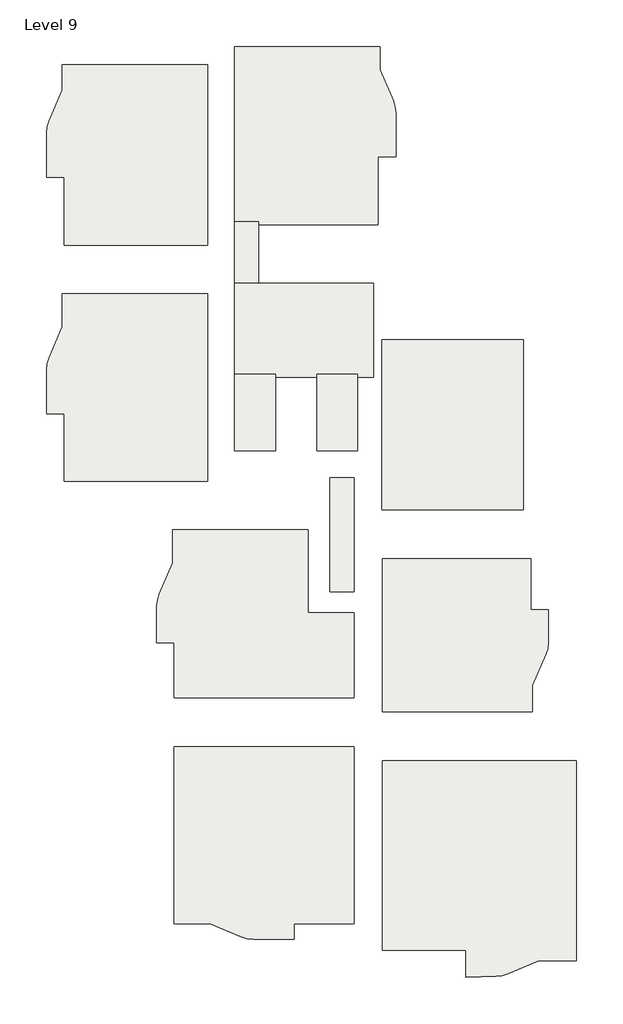
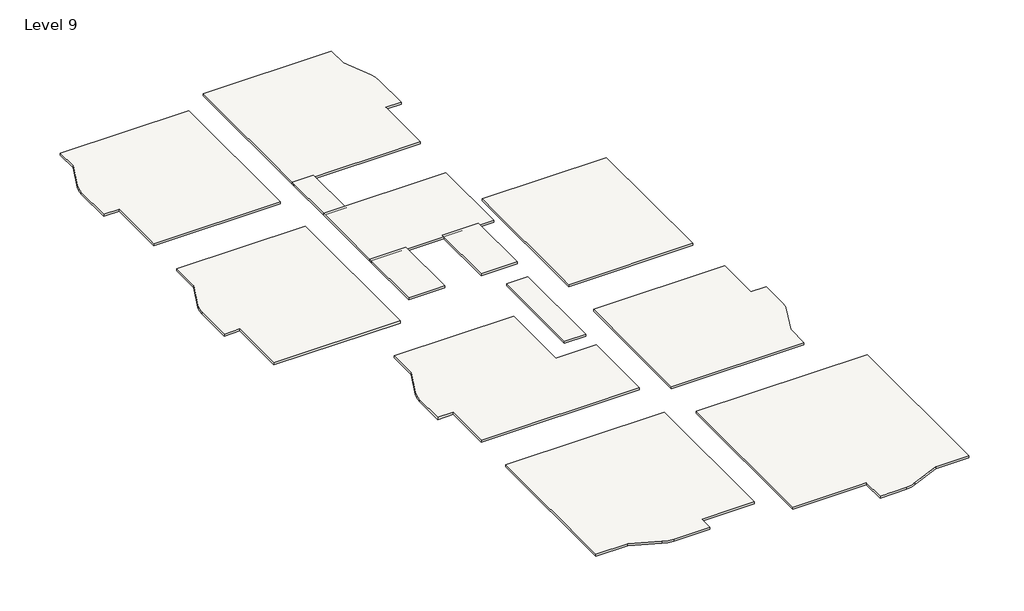
# One storey: 13 roofs.
"""IFC4 building model written with IfcOpenShell, lengths in millimetres."""

from ifc_helpers import new_model, si_unit, point, frame, frame_2d, origin, place, context, project, spatial, polyline, circle_curve, trimmed, segment, composite_curve, outline, extrude, element, save

model = new_model("IFC4")

# Units and contexts
model_context = context("Model", 3, world=origin())
ifc_project = project(units=[si_unit("LENGTHUNIT", "METRE", prefix="MILLI")], contexts=[model_context])

# Site, building, storey
site = spatial("IfcSite", under=ifc_project)
building = spatial("IfcBuilding", under=site)
storey = spatial("IfcBuildingStorey", under=building, Name="Level 9", Elevation=24384.0)

# Roofs
placement = place(None, origin())
element("IfcRoof", 1, ObjectType="Generic - 12\"", at=placement, inside=storey, context=model_context, shape_type="SweptSolid", body=[
    extrude(outline(composite_curve([segment(polyline([(-10024.8708389, -25100.3416506), (-12290.487215, -25100.3416506), (-12290.487215, -13962.4416506), (-986.8891351, -13962.4416506), (-986.8891351, -25100.3416506), (-4746.0891351, -25100.3416506), (-4746.0891351, -26090.9416506), (-7315.6413127, -26090.9416506)]), True, "CONTINUOUS"), segment(trimmed(circle_curve(frame_2d((-7315.6413127, -24160.5416506)), 1930.4), [point((-7315.6413127, -26090.9416506))], [point((-8075.5356374, -25935.0851906))], False, "CARTESIAN"), True, "CONTINUOUS"), segment(polyline([(-8075.5356374, -25935.0851906), (-10024.8708389, -25100.3416506)]), True, "CONTINUOUS")], self_intersect=False)), frame((0.0, 0.0, 24384.0), z_axis=(0.0, 0.0, 1.0), x_axis=(1.0, 0.0, 0.0)), (0.0, 0.0, 1.0), 152.4),
])
element("IfcRoof", 2, ObjectType="Generic - 12\"", at=placement, inside=storey, context=model_context, shape_type="SweptSolid", body=[
    extrude(outline(composite_curve([segment(polyline([(6070.4380523, -26783.9042694), (812.6380523, -26783.9042694), (812.6380523, -14845.9042694), (13017.3380523, -14845.9042694), (13017.3380523, -27431.6042694), (10660.5280667, -27431.6042694), (8711.1928652, -28266.3478094)]), True, "CONTINUOUS"), segment(trimmed(circle_curve(frame_2d((7951.2985405, -26491.8042694)), 1930.4), [point((8711.1928652, -28266.3478094))], [point((7953.0959373, -28422.2034326))], False, "CARTESIAN"), True, "CONTINUOUS"), segment(polyline([(7953.0959373, -28422.2034326), (6070.4380523, -28487.9472947), (6070.4380523, -26783.9042694)]), True, "CONTINUOUS")], self_intersect=False)), frame((0.0, 0.0, 24384.0), z_axis=(0.0, 0.0, 1.0), x_axis=(1.0, 0.0, 0.0)), (0.0, 0.0, 1.0), 152.4),
])
element("IfcRoof", 3, ObjectType="Generic - 12\"", at=placement, inside=storey, context=model_context, shape_type="SweptSolid", body=[
    extrude(outline(composite_curve([segment(polyline([(10274.1380523, -11759.8042694), (803.8108649, -11759.8042694), (803.8108649, -2133.2042694), (10159.8380523, -2133.2042694), (10159.8380523, -5352.6542694), (11264.7380523, -5352.6542694), (11264.7380523, -7397.5810633)]), True, "CONTINUOUS"), segment(trimmed(circle_curve(frame_2d((9334.3380523, -7397.5810633)), 1930.4), [point((11264.7380523, -7397.5810633))], [point((11108.8815923, -8157.475388))], False, "CARTESIAN"), True, "CONTINUOUS"), segment(polyline([(11108.8815923, -8157.475388), (10274.1380523, -10106.8105895), (10274.1380523, -11759.8042694)]), True, "CONTINUOUS")], self_intersect=False)), frame((0.0, 0.0, 24384.0), z_axis=(0.0, 0.0, 1.0), x_axis=(1.0, 0.0, 0.0)), (0.0, 0.0, 1.0), 152.4),
])
element("IfcRoof", 4, ObjectType="Generic - 12\"", at=placement, inside=storey, context=model_context, shape_type="SweptSolid", body=[
    extrude(outline(composite_curve([segment(polyline([(-13395.387215, -7421.9416506), (-13395.387215, -5140.4900045)]), True, "CONTINUOUS"), segment(trimmed(circle_curve(frame_2d((-11464.987215, -5140.4900045)), 1930.4), [point((-13395.387215, -5140.4900045))], [point((-13239.530755, -4380.5956799))], False, "CARTESIAN"), True, "CONTINUOUS"), segment(polyline([(-13239.530755, -4380.5956799), (-12404.787215, -2431.2604783), (-12404.787215, -322.6416506), (-3857.687215, -322.6416506), (-3857.687215, -5523.2916506), (-974.1891351, -5523.2916506), (-974.1891351, -10889.0416506), (-12290.487215, -10889.0416506), (-12290.487215, -7421.9416506), (-13395.387215, -7421.9416506)]), True, "CONTINUOUS")], self_intersect=False)), frame((0.0, 0.0, 24384.0), z_axis=(0.0, 0.0, 1.0), x_axis=(1.0, 0.0, 0.0)), (0.0, 0.0, 1.0), 152.4),
])
element("IfcRoof", 5, ObjectType="Generic - 12\"", at=placement, inside=storey, context=model_context, shape_type="SweptSolid", body=[
    extrude(outline(polyline([(-2472.7891351, 2953.9583494), (-961.4891351, 2953.9583494), (-961.4891351, -4202.4916506), (-2472.7891351, -4202.4916506), (-2472.7891351, 2953.9583494)])), frame((0.0, 0.0, 24384.0), z_axis=(0.0, 0.0, 1.0), x_axis=(1.0, 0.0, 0.0)), (0.0, 0.0, 1.0), 152.4),
])
element("IfcRoof", 6, ObjectType="Generic - 12\"", at=placement, inside=storey, context=model_context, shape_type="SweptSolid", body=[
    extrude(outline(composite_curve([segment(polyline([(-10194.3891351, 2750.7583494), (-19236.7891351, 2750.7583494), (-19236.7891351, 6979.8583494), (-20341.6891351, 6979.8583494), (-20341.6891351, 9746.7948172)]), True, "CONTINUOUS"), segment(trimmed(circle_curve(frame_2d((-18411.2891351, 9746.7948172)), 1930.4), [point((-20341.6891351, 9746.7948172))], [point((-20185.8326751, 10506.6891419))], False, "CARTESIAN"), True, "CONTINUOUS"), segment(polyline([(-20185.8326751, 10506.6891419), (-19351.0891351, 12456.0243434), (-19351.0891351, 14536.3583494), (-10194.3891351, 14536.3583494), (-10194.3891351, 2750.7583494)]), True, "CONTINUOUS")], self_intersect=False)), frame((0.0, 0.0, 24384.0), z_axis=(0.0, 0.0, 1.0), x_axis=(1.0, 0.0, 0.0)), (0.0, 0.0, 1.0), 152.4),
])
element("IfcRoof", 7, ObjectType="Generic - 12\"", at=placement, inside=storey, context=model_context, shape_type="SweptSolid", body=[
    extrude(outline(composite_curve([segment(polyline([(-10194.3891351, 17609.7583494), (-19236.7891351, 17609.7583494), (-19236.7891351, 21889.6583494), (-20341.6891351, 21889.6583494), (-20341.6891351, 24656.5948172)]), True, "CONTINUOUS"), segment(trimmed(circle_curve(frame_2d((-18411.2891351, 24656.5948172)), 1930.4), [point((-20341.6891351, 24656.5948172))], [point((-20185.8326751, 25416.4891419))], False, "CARTESIAN"), True, "CONTINUOUS"), segment(polyline([(-20185.8326751, 25416.4891419), (-19351.0891351, 27365.8243434), (-19351.0891351, 28950.8583494), (-10194.3891351, 28950.8583494), (-10194.3891351, 17609.7583494)]), True, "CONTINUOUS")], self_intersect=False)), frame((0.0, 0.0, 24384.0), z_axis=(0.0, 0.0, 1.0), x_axis=(1.0, 0.0, 0.0)), (0.0, 0.0, 1.0), 152.4),
])
element("IfcRoof", 8, ObjectType="Generic - 12\"", at=placement, inside=storey, context=model_context, shape_type="SweptSolid", body=[
    extrude(outline(composite_curve([segment(polyline([(-8492.5891351, 18875.1215905), (-8492.5891351, 30101.9215905), (664.1108649, 30101.9215905), (664.1108649, 28631.1875845), (1498.8544049, 26681.8523829)]), True, "CONTINUOUS"), segment(trimmed(circle_curve(frame_2d((-275.6891351, 25921.9580583)), 1930.4), [point((1498.8544049, 26681.8523829))], [point((1654.7108649, 25921.9580583))], False, "CARTESIAN"), True, "CONTINUOUS"), segment(polyline([(1654.7108649, 25921.9580583), (1654.7108649, 23155.0215905), (549.8108649, 23155.0215905), (549.8108649, 18875.1215905), (-8492.5891351, 18875.1215905)]), True, "CONTINUOUS")], self_intersect=False)), frame((0.0, 0.0, 24384.0), z_axis=(0.0, 0.0, 1.0), x_axis=(1.0, 0.0, 0.0)), (0.0, 0.0, 1.0), 152.4),
])
element("IfcRoof", 9, ObjectType="Generic - 12\"", at=placement, inside=storey, context=model_context, shape_type="SweptSolid", body=[
    extrude(outline(polyline([(-8492.5891351, 9478.4949943), (-5914.4891351, 9478.4949943), (-5914.4891351, 4665.1949943), (-8492.5891351, 4665.1949943), (-8492.5891351, 9478.4949943)])), frame((0.0, 0.0, 24384.0), z_axis=(0.0, 0.0, 1.0), x_axis=(1.0, 0.0, 0.0)), (0.0, 0.0, 1.0), 152.4),
])
element("IfcRoof", 10, ObjectType="Generic - 12\"", at=placement, inside=storey, context=model_context, shape_type="SweptSolid", body=[
    extrude(outline(polyline([(-3310.9891351, 9478.4949943), (-745.5891351, 9478.4949943), (-745.5891351, 4652.4949943), (-3310.9891351, 4652.4949943), (-3310.9891351, 9478.4949943)])), frame((0.0, 0.0, 24384.0), z_axis=(0.0, 0.0, 1.0), x_axis=(1.0, 0.0, 0.0)), (0.0, 0.0, 1.0), 152.4),
])
element("IfcRoof", 11, ObjectType="Generic - 12\"", at=placement, inside=storey, context=model_context, shape_type="SweptSolid", body=[
    extrude(outline(polyline([(-8492.5891351, 19078.3215905), (-6993.9891351, 19078.3215905), (-6993.9891351, 14988.9215905), (-8492.5891351, 14988.9215905), (-8492.5891351, 19078.3215905)])), frame((0.0, 0.0, 24384.0), z_axis=(0.0, 0.0, 1.0), x_axis=(1.0, 0.0, 0.0)), (0.0, 0.0, 1.0), 152.4),
])
element("IfcRoof", 12, ObjectType="Generic - 12\"", at=placement, inside=storey, context=model_context, shape_type="SweptSolid", body=[
    extrude(outline(polyline([(-8492.5891351, 15192.1215905), (257.7108649, 15192.1215905), (257.7108649, 9275.2949943), (-8492.5891351, 9275.2949943), (-8492.5891351, 15192.1215905)])), frame((0.0, 0.0, 24384.0), z_axis=(0.0, 0.0, 1.0), x_axis=(1.0, 0.0, 0.0)), (0.0, 0.0, 1.0), 152.4),
])
element("IfcRoof", 13, ObjectType="Generic - 12\"", at=placement, inside=storey, context=model_context, shape_type="SweptSolid", body=[
    extrude(outline(polyline([(793.5880523, 11646.2957306), (9677.2380523, 11646.2957306), (9677.2380523, 940.1957306), (793.5880523, 940.1957306), (793.5880523, 11646.2957306)])), frame((0.0, 0.0, 24384.0), z_axis=(0.0, 0.0, 1.0), x_axis=(1.0, 0.0, 0.0)), (0.0, 0.0, 1.0), 152.4),
])

save(model, "model.ifc")

# Revit data of these elements
# Type "Generic - 12\""
#   Assembly Code = "B1020"
#   Layers, outside or top first: 0' - 6" no material (function 1)
# Elements 1, 2, 3, 4, 5, 6, 7, 8, 9, 10, 11, 12, 13 (IfcRoof, "Generic - 12\"")
#   built-in parameter 1001705 = 80.5 (stored number, unit not read)
#   built-in parameter 1001710 = 33615
#   Phase Created = New Construction
#   Materials on its faces: "Default Roof"
# Materials
#   "Default Roof": colour RGB 88 101 114, transparency 0, Cost = 0
